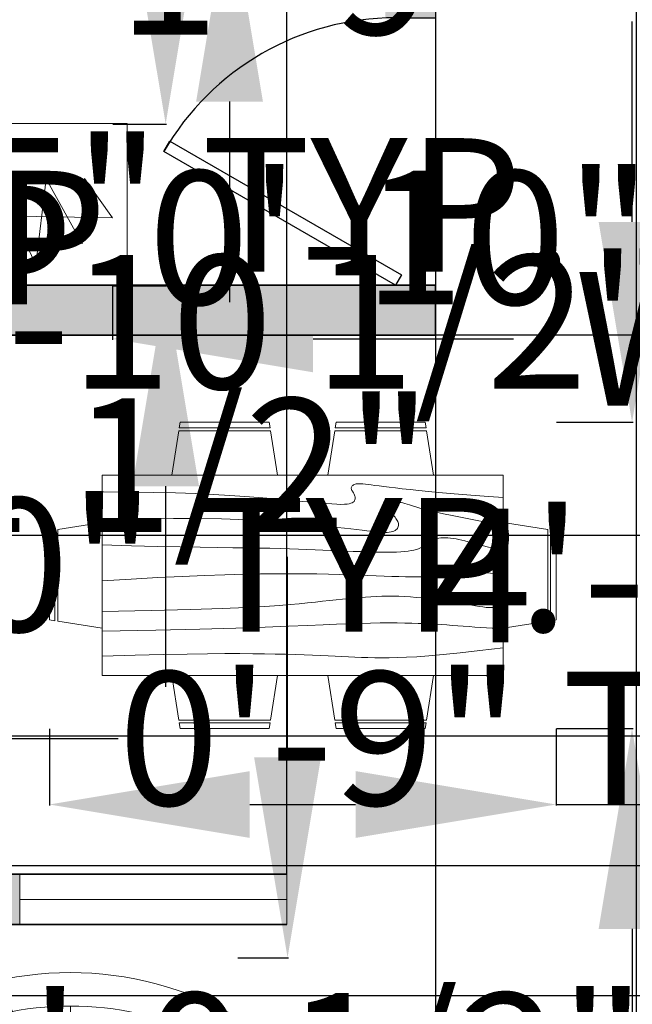
# Model space of a CAD drawing. Units: inches. Extents: x 2838 to 4029, y 1041 to 1915.
# Tile 6 of 16: x 3331 to 3441, y 1377 to 1554. Entities that reach past the tile are written whole.
import ezdxf

# ---------------------------------------------------------------- set-up
doc = ezdxf.new("R2010")
doc.units = ezdxf.units.IN
doc.header["$MEASUREMENT"] = 0
for name, color, linetype, lineweight in [('A-ANNO-DIMS', 2, 'Continuous', 18), ('A-DOOR', 3, 'Continuous', 25), ('A-FLOR-CASE', 8, 'Continuous', 18), ('A-FURN', 8, 'Continuous', 18), ('A-GLAZ', 4, 'Continuous', 18), ('A-WALL', 7, 'Continuous', 35), ('A-WALL-PATT', 252, 'Continuous', 13)]:
    doc.layers.add(name, color=color, linetype=linetype, lineweight=lineweight)
doc.styles.get("Standard").update_dxf_attribs({"font": 'arial.ttf'})
doc.dimstyles.get("Standard").update_dxf_attribs({"dimtxt": 24, "dimasz": 36, "dimexe": 0.18, "dimexo": 0.0625, "dimgap": 0.09, "dimtad": 0, "dimtih": 1, "dimtoh": 1, "dimdec": 0, "dimzin": 0, "dimdsep": 46, "dimlunit": 3, "dimtxsty": 'Standard', "dimcen": 0.09, "dimadec": 0, "dimazin": 0, "dimtfac": 1, "dimtdec": 0, "dimtofl": 0, "dimtmove": 0, "dimatfit": 3, "dimfxl": 1, "dimtolj": 1, "dimtzin": 0, "dimarcsym": 0})

# ---------------------------------------------------------------- blocks, each defined once
blk = doc.blocks.new('*U3')
for p, q in [((-40, 0), (-40, 6)), ((0, 0), (0, 6))]:
    blk.add_line(p, q)
blk.add_lwpolyline([(0, 0), (-20, -34.64), (-21.52, -33.77), (-1.52, 0.88)], close=True)
blk.add_arc((0, 0), 40, 180, 240)
blk = doc.blocks.new('Sofa - Roundback Loveseat 5 ft.')
for p, q in [((0, -32.44198), (0, -5.99998)), ((-24, -33.99998), (-24, -11.46958)), ((24.00004, -33.99998), (24.00004, -11.46958)), ((-23.9998, -13.38178), (23.99986, -13.38178)), ((-24, -32.44198), (24.00004, -32.44198))]:
    blk.add_line(p, q)
for points in [[(-24, -33.99998), (-30, -33.99998), (-30, -7.99998)], [(30.00004, -7.99998), (30.00004, -33.99998), (24.00004, -33.99998)]]:
    blk.add_lwpolyline(points)
for centre, radius, start, end in [((0, -60.24998), 60.24998, 60.13715, 119.8628), ((0, -61.38438), 55.38444, 64.32083, 115.6792)]:
    blk.add_arc(centre, radius, start, end)
blk = doc.blocks.new('Dining Set - 36 x 72 in.')
for p, q in [((-22, 27.5), (-22.1562, 26.50042)), ((-22, 27.5), (-6, 27.5)), ((-5.8437, 26.49966), (-6, 27.5)), ((6, 27.5), (5.8438, 26.50042)), ((6, 27.5), (22, 27.5)), ((22.1563, 26.49966), (22, 27.5)), ((-22.2343, 26.00059), (-23.4847, 17.99762)), ((-22.2304, 26), (-5.7608, 26)), ((-5.8416, 26.5), (-22.1534, 26.5)), ((-4.5152, 17.99762), (-5.7655, 25.99926)), ((5.7657, 26.00059), (4.5153, 17.99762)), ((5.7696, 26), (22.2392, 26)), ((22.1584, 26.5), (5.8466, 26.5)), ((23.4848, 17.99762), (22.2345, 25.99926)), ((36, 18), (-36, 18)), ((-36, 18), (-36, -18)), ((36, -18), (36, 18)), ((-44.0006, 8.23428), (-35.9976, 9.48474)), ((44.0006, 8.23428), (35.9976, 9.48474)), ((-45.5, 8), (-44.5004, 8.15617)), ((-45.5, 8), (-45.5, -8)), ((-44.5, -8.15843), (-44.5, 8.15338)), ((-44, 8.23041), (-44, -8.23915)), ((44, 8.23041), (44, -8.23915)), ((44.5, -8.15843), (44.5, 8.15338)), ((45.5, 8), (44.5005, 8.15617)), ((45.5, 8), (45.5, -8)), ((-44.4997, -8.15631), (-45.5, -8)), ((-35.9976, -9.48476), (-43.9993, -8.2345)), ((35.9976, -9.48476), (43.9993, -8.2345)), ((44.4997, -8.15631), (45.5, -8)), ((-36, -18), (36, -18)), ((-22.2343, -26.0006), (-23.4847, -17.99762)), ((-4.5152, -17.99762), (-5.7655, -25.99928)), ((5.7657, -26.0006), (4.5153, -17.99762)), ((23.4848, -17.99762), (22.2345, -25.99928)), ((-22.2304, -26), (-5.7608, -26)), ((-22, -27.5), (-22.1562, -26.50044)), ((-5.8416, -26.5), (-22.1534, -26.5)), ((-5.8437, -26.49967), (-6, -27.5)), ((5.7696, -26), (22.2392, -26)), ((6, -27.5), (5.8438, -26.50044)), ((22.1584, -26.5), (5.8466, -26.5)), ((22.1563, -26.49967), (22, -27.5)), ((-22, -27.5), (-6, -27.5)), ((6, -27.5), (22, -27.5))]:
    blk.add_line(p, q)
for points in [[(-36, 15), (-31.1772, 14.97754), (-26.8079, 14.91406), (-22.8538, 14.81543), (-19.276, 14.6875), (-16.0362, 14.53613), (-13.0957, 14.36718), (-10.4159, 14.18652), (-7.9583, 14), (-5.6904, 13.81315), (-3.6035, 13.63021), (-1.6954, 13.45508), (0.0365, 13.29166), (1.5945, 13.14388), (2.9811, 13.01562), (4.1988, 12.9108), (5.25, 12.83333), (6.1393, 12.78613), (6.8802, 12.76823), (7.4883, 12.77767), (7.9792, 12.8125), (8.3685, 12.87077), (8.6719, 12.95052), (8.9049, 13.0498), (9.0833, 13.16666), (9.2205, 13.29899), (9.3216, 13.44401), (9.3895, 13.59879), (9.4271, 13.76041), (9.4373, 13.92594), (9.4232, 14.09245), (9.3875, 14.257), (9.3333, 14.41666), (9.2638, 14.56917), (9.1836, 14.71484), (9.0975, 14.85465), (9.0104, 14.98958), (8.9272, 15.1206), (8.8529, 15.2487), (8.7922, 15.37483), (8.75, 15.5), (8.7305, 15.62467), (8.7344, 15.74739), (8.7617, 15.86621), (8.8125, 15.97916), (8.8867, 16.08431), (8.9844, 16.17968), (9.1055, 16.26334), (9.25, 16.33333), (9.4189, 16.38802), (9.6172, 16.42708), (9.8506, 16.45052), (10.125, 16.45833), (10.4463, 16.45052), (10.8203, 16.42708), (11.2529, 16.38802), (11.75, 16.33333), (12.3184, 16.26318), (12.9694, 16.17838), (13.7151, 16.07991), (14.5677, 15.96875), (15.5395, 15.84586), (16.6426, 15.71224), (17.8893, 15.56884), (19.2917, 15.41666), (20.859, 15.25667), (22.5879, 15.08984), (24.4721, 14.91715), (26.5052, 14.73958), (28.6809, 14.5581), (30.9929, 14.3737), (33.4347, 14.18733), (36, 14)], [(-36, 10), (-28.9766, 10.14274), (-23.1725, 10.20442), (-18.4241, 10.19775), (-14.5677, 10.13541), (-11.4399, 10.03011), (-8.877, 9.89453), (-6.7154, 9.74137), (-4.7917, 9.58333), (-2.9698, 9.43082), (-1.2246, 9.28515), (0.4415, 9.14534), (2.026, 9.01041), (3.5266, 8.87939), (4.9408, 8.7513), (6.266, 8.62516), (7.5, 8.5), (8.6411, 8.37549), (9.6914, 8.2539), (10.6538, 8.13818), (11.5312, 8.03125), (12.3267, 7.93603), (13.043, 7.85547), (13.6831, 7.79248), (14.25, 7.75), (14.7471, 7.7303), (15.1797, 7.73307), (15.5537, 7.75732), (15.875, 7.80208), (16.1494, 7.86637), (16.3828, 7.94922), (16.5811, 8.04964), (16.75, 8.16666), (16.8944, 8.29915), (17.0143, 8.44531), (17.1089, 8.60319), (17.1771, 8.77083), (17.218, 8.94629), (17.2305, 9.1276), (17.2137, 9.31282), (17.1667, 9.5), (17.0895, 9.6875), (16.987, 9.875), (16.8649, 10.0625), (16.7292, 10.25), (16.5856, 10.4375), (16.4401, 10.625), (16.2985, 10.8125), (16.1667, 11), (16.05, 11.18733), (15.9518, 11.3737), (15.8752, 11.5581), (15.8229, 11.73958), (15.798, 11.91715), (15.8034, 12.08984), (15.842, 12.25667), (15.9167, 12.41666), (16.0295, 12.56836), (16.1784, 12.70833), (16.3605, 12.83268), (16.5729, 12.9375), (16.8127, 13.01888), (17.0768, 13.07291), (17.3625, 13.0957), (17.6667, 13.08333), (17.9894, 13.03312), (18.3418, 12.94726), (18.7382, 12.82918), (19.1927, 12.68229), (19.7195, 12.51001), (20.3327, 12.31575), (21.0465, 12.10294), (21.875, 11.875), (22.8357, 11.63354), (23.959, 11.37304), (25.2786, 11.08618), (26.8282, 10.76562), (28.6414, 10.40405), (30.752, 9.99414), (33.1936, 9.52856), (36, 9)], [(-36, 5.5), (-30.7157, 5.3348), (-26.069, 5.20963), (-21.9946, 5.11767), (-18.4271, 5.05208), (-15.3009, 5.00602), (-12.5508, 4.97265), (-10.1112, 4.94515), (-7.9167, 4.91666), (-5.909, 4.88167), (-4.0586, 4.83984), (-2.3429, 4.79215), (-0.7396, 4.73958), (0.7739, 4.6831), (2.22, 4.6237), (3.6213, 4.56233), (5, 4.5), (6.373, 4.43782), (7.7344, 4.3776), (9.0723, 4.32129), (10.375, 4.27083), (11.6309, 4.22819), (12.8281, 4.19531), (13.9551, 4.17415), (15, 4.16666), (15.954, 4.17448), (16.819, 4.19791), (17.6001, 4.23698), (18.3021, 4.29166), (18.9299, 4.36198), (19.4883, 4.44791), (19.9823, 4.54948), (20.4167, 4.66666), (20.7969, 4.79899), (21.1302, 4.94401), (21.4245, 5.09879), (21.6875, 5.26041), (21.9271, 5.42594), (22.1511, 5.59245), (22.3672, 5.757), (22.5834, 5.91666), (22.8065, 6.06868), (23.0404, 6.21093), (23.2879, 6.34147), (23.5521, 6.45833), (23.8358, 6.55957), (24.142, 6.64323), (24.4735, 6.70735), (24.8334, 6.75), (25.2235, 6.76969), (25.642, 6.76692), (26.0858, 6.74267), (26.5521, 6.69791), (27.0379, 6.63362), (27.5404, 6.55078), (28.0565, 6.45036), (28.5834, 6.33333), (29.1242, 6.19987), (29.7071, 6.04687), (30.3661, 5.87044), (31.1354, 5.66666), (32.0493, 5.43164), (33.142, 5.16146), (34.4475, 4.85221), (36, 4.5)], [(-36, -1), (-30.7915, -0.6591), (-26.0195, -0.38216), (-21.6519, -0.16284), (-17.6563, 0.00521), (-14.0005, 0.12833), (-10.6523, 0.21289), (-7.5796, 0.26522), (-4.75, 0.29166), (-2.134, 0.29793), (0.2878, 0.28711), (2.5317, 0.26163), (4.6146, 0.22396), (6.5529, 0.17651), (8.3633, 0.12174), (10.0623, 0.06209), (11.6667, 0), (13.1899, -0.06201), (14.6341, -0.1211), (15.9982, -0.17432), (17.2813, -0.21875), (18.4823, -0.25147), (19.6003, -0.26953), (20.6343, -0.27002), (21.5834, -0.25), (22.4481, -0.20768), (23.2357, -0.14584), (23.9549, -0.06836), (24.6146, 0.02083), (25.2235, 0.11784), (25.7904, 0.21875), (26.3241, 0.31966), (26.8334, 0.41666), (27.3265, 0.50618), (27.8099, 0.58593), (28.2894, 0.65397), (28.7709, 0.70833), (29.2601, 0.74707), (29.763, 0.76823), (30.2855, 0.76985), (30.8334, 0.75), (31.4088, 0.70784), (31.9994, 0.64713), (32.589, 0.57275), (33.1615, 0.48958), (33.7008, 0.4025), (34.1908, 0.3164), (34.6153, 0.23616), (34.9584, 0.16666), (35.2099, 0.11165), (35.3848, 0.07031), (35.504, 0.04069), (35.5886, 0.02083), (35.6594, 0.00879), (35.7377, 0.0026), (35.8442, 0.00032), (36, 0)], [(-36, -6.5), (-27.1843, -6.31267), (-20.084, -6.1263), (-14.469, -5.9419), (-10.1094, -5.76042), (-6.7752, -5.58285), (-4.2363, -5.41016), (-2.2629, -5.24333), (-0.625, -5.08334), (0.8708, -4.93099), (2.2715, -4.78646), (3.5872, -4.64974), (4.8281, -4.52084), (6.0046, -4.39974), (7.127, -4.28646), (8.2053, -4.18099), (9.25, -4.08334), (10.2705, -3.99382), (11.2734, -3.91407), (12.2647, -3.84603), (13.25, -3.79167), (14.2354, -3.75293), (15.2266, -3.73177), (16.2295, -3.73015), (17.25, -3.75), (18.2912, -3.79248), (19.3451, -3.85547), (20.4009, -3.93604), (21.4479, -4.03125), (22.4754, -4.13819), (23.4727, -4.25391), (24.4289, -4.37549), (25.3334, -4.5), (26.1785, -4.62492), (26.9694, -4.74935), (27.7145, -4.87281), (28.4219, -4.99479), (29.1, -5.11483), (29.7572, -5.23242), (30.4016, -5.34709), (31.0417, -5.45834), (31.6837, -5.56437), (32.3262, -5.65821), (32.9658, -5.73153), (33.599, -5.77604), (34.2224, -5.78345), (34.8327, -5.74545), (35.4264, -5.65373), (36, -5.5)], [(-36, -10), (-26.4022, -9.81299), (-18.4675, -9.62891), (-11.9839, -9.45069), (-6.7396, -9.28125), (-2.5226, -9.12354), (0.8789, -8.98047), (3.6769, -8.85498), (6.0833, -8.75), (8.2767, -8.66765), (10.3021, -8.60677), (12.1712, -8.56543), (13.8958, -8.54167), (15.4876, -8.53353), (16.9583, -8.53907), (18.3197, -8.55632), (19.5834, -8.58334), (20.7616, -8.61841), (21.8685, -8.66081), (22.9188, -8.71004), (23.9271, -8.76563), (24.9081, -8.82707), (25.8763, -8.89388), (26.8465, -8.96558), (27.8334, -9.04167), (28.8474, -9.12118), (29.8828, -9.20117), (30.93, -9.27824), (31.9792, -9.34896), (33.0205, -9.40991), (34.0443, -9.45768), (35.0407, -9.48885), (36, -9.5)], [(-36, -14.5), (-30.0881, -14.33513), (-25.0332, -14.21224), (-20.7312, -14.12647), (-17.0781, -14.07292), (-13.97, -14.04671), (-11.3027, -14.04297), (-8.9724, -14.05681), (-6.875, -14.08334), (-4.9224, -14.11833), (-3.0905, -14.16016), (-1.3709, -14.20785), (0.2448, -14.26042), (1.7647, -14.3169), (3.1973, -14.3763), (4.5507, -14.43767), (5.8333, -14.5), (7.0554, -14.5621), (8.235, -14.62175), (9.3922, -14.67652), (10.5469, -14.72396), (11.7192, -14.76164), (12.929, -14.78711), (14.1965, -14.79794), (15.5417, -14.79167), (16.9933, -14.76424), (18.6152, -14.70508), (20.4804, -14.60197), (22.6615, -14.44271), (25.2312, -14.21509), (28.2624, -13.9069), (31.8277, -13.50594), (36, -13)]]:
    blk.add_lwpolyline(points)
blk = doc.blocks.new('WIN-48')
blk.add_line((4.5, 48), (4.5, 0))
blk.add_lwpolyline([(0, 48), (9, 48), (9, 0), (0, 0)], close=True)
blk = doc.blocks.new('WARDROBE-RAIL')
for p, q in [((1.86, 0), (12.76, 29.05)), ((12.76, 29.05), (12.76, 0)), ((12.76, 0), (20.9, 24.31)), ((20.9, 24.31), (26.94, 1.83)), ((26.94, 1.83), (31.9, 21.29)), ((31.9, 21.29), (40.3, 2.75)), ((40.3, 2.75), (41.22, 21.97)), ((41.22, 21.97), (49.7, 3.76)), ((1.8, 18), (1.86, 0)), ((49.7, 3.76), (51.56, 19.2)), ((51.56, 19.2), (58.03, 7.54)), ((58.03, 7.54), (58.45, 19.29)), ((58.45, 19.29), (63.49, 12.24)), ((63.49, 12.24), (0, 13.24)), ((0, 13.24), (63.49, 12.24))]:
    blk.add_line(p, q)
blk = doc.blocks.new('*D25')
at = {"layer": 'A-ANNO-DIMS', "color": 0, "lineweight": -2, "transparency": 16777216}
for p, q in [((3283.93, 1516.17), (3283.93, 1552.17)), ((3276.79, 1480.17), (3284.11, 1480.17)), ((3276.79, 1432.17), (3284.11, 1432.17)), ((3283.93, 1396.17), (3283.93, 1360.17))]:
    blk.add_line(p, q, dxfattribs=at)
at = {"layer": 'A-ANNO-DIMS', "color": 0, "transparency": 16777216}
for points in [[(3277.93, 1516.17), (3289.93, 1516.17), (3283.93, 1480.17)], [(3277.93, 1396.17), (3289.93, 1396.17), (3283.93, 1432.17)]]:
    blk.add_solid(points, dxfattribs=at)
at = {"layer": 'Defpoints', "color": 0, "transparency": 16777216}
for p in [(3276.73, 1480.17), (3283.93, 1480.17), (3276.73, 1432.17)]:
    blk.add_point(p, dxfattribs=at)
at = {"layer": 'A-ANNO-DIMS', "color": 0, "transparency": 16777216, "insert": (3283.93, 1456.17), "char_height": 24, "attachment_point": 5}
blk.add_mtext('\\A1;WINDOW 4\'-0" TYP.', dxfattribs=at)
blk = doc.blocks.new('*D26')
at = {"layer": 'A-ANNO-DIMS', "color": 0, "lineweight": -2, "transparency": 16777216}
for p, q in [((3267.73, 1432.1), (3267.73, 1424.79)), ((3276.73, 1432.1), (3276.73, 1424.79)), ((3231.73, 1424.97), (3195.73, 1424.97)), ((3312.73, 1424.97), (3348.73, 1424.97))]:
    blk.add_line(p, q, dxfattribs=at)
at = {"layer": 'A-ANNO-DIMS', "color": 0, "transparency": 16777216}
for points in [[(3231.73, 1430.97), (3231.73, 1418.97), (3267.73, 1424.97)], [(3312.73, 1430.97), (3312.73, 1418.97), (3276.73, 1424.97)]]:
    blk.add_solid(points, dxfattribs=at)
at = {"layer": 'Defpoints', "color": 0, "transparency": 16777216}
for p in [(3267.73, 1432.17), (3276.73, 1432.17), (3276.73, 1424.97)]:
    blk.add_point(p, dxfattribs=at)
at = {"layer": 'A-ANNO-DIMS', "color": 0, "transparency": 16777216, "insert": (3421.97, 1424.97), "char_height": 24, "attachment_point": 5}
blk.add_mtext('\\A1;0\'-9" TYP.', dxfattribs=at)
blk = doc.blocks.new('*D30')
at = {"layer": 'A-ANNO-DIMS', "color": 0, "lineweight": -2, "transparency": 16777216}
for p, q in [((3379.15, 1421.58), (3379.15, 1457.58)), ((3370.21, 1385.58), (3379.33, 1385.58)), ((3370.21, 1348.91), (3379.33, 1348.91)), ((3379.15, 1312.91), (3379.15, 1276.91))]:
    blk.add_line(p, q, dxfattribs=at)
at = {"layer": 'A-ANNO-DIMS', "color": 0, "transparency": 16777216}
for points in [[(3373.15, 1421.58), (3385.15, 1421.58), (3379.15, 1385.58)], [(3373.15, 1312.91), (3385.15, 1312.91), (3379.15, 1348.91)]]:
    blk.add_solid(points, dxfattribs=at)
at = {"layer": 'Defpoints', "color": 0, "transparency": 16777216}
for p in [(3370.15, 1385.58), (3379.15, 1385.58), (3370.15, 1348.91)]:
    blk.add_point(p, dxfattribs=at)
at = {"layer": 'A-ANNO-DIMS', "color": 0, "transparency": 16777216, "insert": (3379.15, 1367.25), "char_height": 24, "attachment_point": 5}
blk.add_mtext('\\A1;3\'-0 1/2"', dxfattribs=at)
blk = doc.blocks.new('*D33')
at = {"layer": 'A-ANNO-DIMS', "color": 0, "lineweight": -2, "transparency": 16777216}
for p, q in [((3601.73, 1469.45), (3601.73, 1505.45)), ((3603.48, 1433.45), (3601.55, 1433.45)), ((3603.48, 1421.37), (3601.55, 1421.37)), ((3601.73, 1385.37), (3601.73, 1349.37)), ((3601.73, 1349.37), (3565.73, 1349.37))]:
    blk.add_line(p, q, dxfattribs=at)
at = {"layer": 'A-ANNO-DIMS', "color": 0, "transparency": 16777216}
for points in [[(3595.73, 1469.45), (3607.73, 1469.45), (3601.73, 1433.45)], [(3595.73, 1385.37), (3607.73, 1385.37), (3601.73, 1421.37)]]:
    blk.add_solid(points, dxfattribs=at)
at = {"layer": 'Defpoints', "color": 0, "transparency": 16777216}
for p in [(3603.54, 1433.45), (3601.73, 1421.37), (3603.54, 1421.37)]:
    blk.add_point(p, dxfattribs=at)
at = {"layer": 'A-ANNO-DIMS', "color": 0, "transparency": 16777216, "insert": (3496.18, 1349.37), "char_height": 24, "attachment_point": 5}
blk.add_mtext('\\A1;TAP 1\'-0"', dxfattribs=at)
blk = doc.blocks.new('*D35')
at = {"layer": 'A-ANNO-DIMS', "color": 0, "lineweight": -2, "transparency": 16777216}
for p, q in [((3480.45, 1632.93), (3480.45, 1668.93)), ((3481.89, 1596.93), (3480.27, 1596.93)), ((3481.89, 1586.93), (3480.27, 1586.93)), ((3480.45, 1550.93), (3480.45, 1514.93)), ((3480.45, 1514.93), (3444.45, 1514.93))]:
    blk.add_line(p, q, dxfattribs=at)
at = {"layer": 'A-ANNO-DIMS', "color": 0, "transparency": 16777216}
for points in [[(3474.45, 1632.93), (3486.45, 1632.93), (3480.45, 1596.93)], [(3474.45, 1550.93), (3486.45, 1550.93), (3480.45, 1586.93)]]:
    blk.add_solid(points, dxfattribs=at)
at = {"layer": 'Defpoints', "color": 0, "transparency": 16777216}
for p in [(3481.95, 1596.93), (3480.45, 1586.93), (3481.95, 1586.93)]:
    blk.add_point(p, dxfattribs=at)
at = {"layer": 'A-ANNO-DIMS', "color": 0, "transparency": 16777216, "insert": (3365.58, 1514.93), "char_height": 24, "attachment_point": 5}
blk.add_mtext('\\A1;TAP 0\'-10"', dxfattribs=at)
blk = doc.blocks.new('*D36')
at = {"layer": 'A-ANNO-DIMS', "color": 0, "lineweight": -2, "transparency": 16777216}
for p, q in [((3481.95, 1586.87), (3481.95, 1585.25)), ((3488.45, 1586.87), (3488.45, 1585.25)), ((3445.95, 1585.43), (3409.95, 1585.43)), ((3524.45, 1585.43), (3560.45, 1585.43))]:
    blk.add_line(p, q, dxfattribs=at)
at = {"layer": 'A-ANNO-DIMS', "color": 0, "transparency": 16777216}
for points in [[(3445.95, 1591.43), (3445.95, 1579.43), (3481.95, 1585.43)], [(3524.45, 1591.43), (3524.45, 1579.43), (3488.45, 1585.43)]]:
    blk.add_solid(points, dxfattribs=at)
at = {"layer": 'Defpoints', "color": 0, "transparency": 16777216}
for p in [(3481.95, 1586.93), (3488.45, 1586.93), (3488.45, 1585.43)]:
    blk.add_point(p, dxfattribs=at)
at = {"layer": 'A-ANNO-DIMS', "color": 0, "transparency": 16777216, "insert": (3620.4, 1585.43), "char_height": 24, "attachment_point": 5}
blk.add_mtext('\\A1;0\'-6 1/2"', dxfattribs=at)
blk = doc.blocks.new('*D38')
at = {"layer": 'A-ANNO-DIMS', "color": 0, "lineweight": -2, "transparency": 16777216}
for p, q in [((3368.73, 1671.36), (3368.73, 1707.36)), ((3356.79, 1635.36), (3368.91, 1635.36)), ((3356.79, 1575.36), (3368.91, 1575.36)), ((3368.73, 1539.36), (3368.73, 1503.36))]:
    blk.add_line(p, q, dxfattribs=at)
at = {"layer": 'A-ANNO-DIMS', "color": 0, "transparency": 16777216}
for points in [[(3362.73, 1671.36), (3374.73, 1671.36), (3368.73, 1635.36)], [(3362.73, 1539.36), (3374.73, 1539.36), (3368.73, 1575.36)]]:
    blk.add_solid(points, dxfattribs=at)
at = {"layer": 'Defpoints', "color": 0, "transparency": 16777216}
for p in [(3356.73, 1635.36), (3368.73, 1635.36), (3356.73, 1575.36)]:
    blk.add_point(p, dxfattribs=at)
at = {"layer": 'A-ANNO-DIMS', "color": 0, "transparency": 16777216, "insert": (3368.73, 1605.36), "char_height": 24, "attachment_point": 5}
blk.add_mtext('\\A1;5\'-0" TYP.', dxfattribs=at)
blk = doc.blocks.new('*D41')
at = {"layer": 'A-ANNO-DIMS', "color": 0, "lineweight": -2, "transparency": 16777216}
for p, q in [((3284.24, 1506.2), (3284.24, 1496.56)), ((3347.73, 1506.2), (3347.73, 1496.56)), ((3248.24, 1496.74), (3212.24, 1496.74)), ((3383.73, 1496.74), (3419.73, 1496.74))]:
    blk.add_line(p, q, dxfattribs=at)
at = {"layer": 'A-ANNO-DIMS', "color": 0, "transparency": 16777216}
for points in [[(3248.24, 1502.74), (3248.24, 1490.74), (3284.24, 1496.74)], [(3383.73, 1502.74), (3383.73, 1490.74), (3347.73, 1496.74)]]:
    blk.add_solid(points, dxfattribs=at)
at = {"layer": 'Defpoints', "color": 0, "transparency": 16777216}
for p in [(3284.24, 1506.26), (3347.73, 1506.26), (3347.73, 1496.74)]:
    blk.add_point(p, dxfattribs=at)
at = {"layer": 'A-ANNO-DIMS', "color": 0, "transparency": 16777216, "insert": (3624.81, 1496.74), "char_height": 24, "attachment_point": 5}
blk.add_mtext('\\A1;WARDROBE 5\'-3 1/2" TYP.', dxfattribs=at)
blk = doc.blocks.new('*D42')
at = {"layer": 'A-ANNO-DIMS', "color": 0, "lineweight": -2, "transparency": 16777216}
for p, q in [((3357.26, 1571.32), (3357.26, 1607.32)), ((3347.8, 1535.32), (3357.44, 1535.32)), ((3347.8, 1506.26), (3357.44, 1506.26)), ((3357.26, 1470.26), (3357.26, 1434.26))]:
    blk.add_line(p, q, dxfattribs=at)
at = {"layer": 'A-ANNO-DIMS', "color": 0, "transparency": 16777216}
for points in [[(3351.26, 1571.32), (3363.26, 1571.32), (3357.26, 1535.32)], [(3351.26, 1470.26), (3363.26, 1470.26), (3357.26, 1506.26)]]:
    blk.add_solid(points, dxfattribs=at)
at = {"layer": 'Defpoints', "color": 0, "transparency": 16777216}
for p in [(3347.73, 1535.32), (3357.26, 1535.32), (3347.73, 1506.26)]:
    blk.add_point(p, dxfattribs=at)
at = {"layer": 'A-ANNO-DIMS', "color": 0, "transparency": 16777216, "insert": (3357.26, 1520.79), "char_height": 24, "attachment_point": 5}
blk.add_mtext('\\A1;2\'-5" TYP.', dxfattribs=at)
blk = doc.blocks.new('*D46')
at = {"layer": 'A-ANNO-DIMS', "color": 0, "lineweight": -2, "transparency": 16777216}
for p, q in [((3451.73, 1692.41), (3451.73, 1728.41)), ((3456.62, 1656.41), (3451.55, 1656.41)), ((3456.62, 1635.41), (3451.55, 1635.41)), ((3451.73, 1599.41), (3451.73, 1563.41)), ((3451.73, 1563.41), (3415.73, 1563.41))]:
    blk.add_line(p, q, dxfattribs=at)
at = {"layer": 'A-ANNO-DIMS', "color": 0, "transparency": 16777216}
for points in [[(3445.73, 1692.41), (3457.73, 1692.41), (3451.73, 1656.41)], [(3445.73, 1599.41), (3457.73, 1599.41), (3451.73, 1635.41)]]:
    blk.add_solid(points, dxfattribs=at)
at = {"layer": 'Defpoints', "color": 0, "transparency": 16777216}
for p in [(3456.69, 1656.41), (3451.73, 1635.41), (3456.69, 1635.41)]:
    blk.add_point(p, dxfattribs=at)
at = {"layer": 'A-ANNO-DIMS', "color": 0, "transparency": 16777216, "insert": (3384.87, 1563.41), "char_height": 24, "attachment_point": 5}
blk.add_mtext('\\A1;1\'-9"', dxfattribs=at)
blk = doc.blocks.new('*D49')
at = {"layer": 'A-ANNO-DIMS', "color": 0, "lineweight": -2, "transparency": 16777216}
for p, q in [((3336.37, 1426.68), (3336.37, 1412.92)), ((3427.37, 1426.68), (3427.37, 1412.92)), ((3372.37, 1413.1), (3391.37, 1413.1)), ((3427.37, 1413.1), (3463.37, 1413.1))]:
    blk.add_line(p, q, dxfattribs=at)
at = {"layer": 'A-ANNO-DIMS', "color": 0, "transparency": 16777216}
for points in [[(3372.37, 1419.1), (3372.37, 1407.1), (3336.37, 1413.1)], [(3391.37, 1419.1), (3391.37, 1407.1), (3427.37, 1413.1)]]:
    blk.add_solid(points, dxfattribs=at)
at = {"layer": 'Defpoints', "color": 0, "transparency": 16777216}
for p in [(3336.37, 1426.75), (3427.37, 1426.75), (3427.37, 1413.1)]:
    blk.add_point(p, dxfattribs=at)
at = {"layer": 'A-ANNO-DIMS', "color": 0, "transparency": 16777216, "insert": (3595.36, 1413.1), "char_height": 24, "attachment_point": 5}
blk.add_mtext('\\A1;DINING SET 7\'-7"', dxfattribs=at)
blk = doc.blocks.new('*D50')
at = {"layer": 'A-ANNO-DIMS', "color": 0, "lineweight": -2, "transparency": 16777216}
for p, q in [((3441.02, 1517.75), (3441.02, 1553.75)), ((3427.44, 1481.75), (3441.2, 1481.75)), ((3427.44, 1426.75), (3441.2, 1426.75)), ((3441.02, 1390.75), (3441.02, 1354.75))]:
    blk.add_line(p, q, dxfattribs=at)
at = {"layer": 'A-ANNO-DIMS', "color": 0, "transparency": 16777216}
for points in [[(3435.02, 1517.75), (3447.02, 1517.75), (3441.02, 1481.75)], [(3435.02, 1390.75), (3447.02, 1390.75), (3441.02, 1426.75)]]:
    blk.add_solid(points, dxfattribs=at)
at = {"layer": 'Defpoints', "color": 0, "transparency": 16777216}
for p in [(3427.37, 1481.75), (3441.02, 1481.75), (3427.37, 1426.75)]:
    blk.add_point(p, dxfattribs=at)
at = {"layer": 'A-ANNO-DIMS', "color": 0, "transparency": 16777216, "insert": (3441.02, 1454.25), "char_height": 24, "attachment_point": 5}
blk.add_mtext('\\A1;4\'-7"', dxfattribs=at)
blk = doc.blocks.new('*D55')
at = {"layer": 'A-ANNO-DIMS', "color": 0, "lineweight": -2, "transparency": 16777216}
for p, q in [((3491.76, 1499.78), (3455.76, 1499.78)), ((3527.76, 1494.67), (3527.76, 1499.96)), ((3562.26, 1494.67), (3562.26, 1499.96)), ((3598.26, 1499.78), (3634.26, 1499.78))]:
    blk.add_line(p, q, dxfattribs=at)
at = {"layer": 'A-ANNO-DIMS', "color": 0, "transparency": 16777216}
for points in [[(3491.76, 1505.78), (3491.76, 1493.78), (3527.76, 1499.78)], [(3598.26, 1505.78), (3598.26, 1493.78), (3562.26, 1499.78)]]:
    blk.add_solid(points, dxfattribs=at)
at = {"layer": 'Defpoints', "color": 0, "transparency": 16777216}
for p in [(3527.76, 1499.78), (3527.76, 1494.6), (3562.26, 1494.6)]:
    blk.add_point(p, dxfattribs=at)
at = {"layer": 'A-ANNO-DIMS', "color": 0, "transparency": 16777216, "insert": (3260.33, 1499.78), "char_height": 24, "attachment_point": 5}
blk.add_mtext('\\A1;BASE CABINET 2\'-10 1/2"', dxfattribs=at)
blk = doc.blocks.new('*D73')
at = {"layer": 'A-ANNO-DIMS', "color": 0, "lineweight": -2, "transparency": 16777216}
for p, q in [((3425.038746, 1711.522346), (3389.038746, 1711.522346)), ((3461.038746, 1200.359846), (3461.038746, 1711.702346)), ((3618.731626, 1200.359846), (3618.731626, 1711.702346)), ((3654.731626, 1711.522346), (3690.731626, 1711.522346))]:
    blk.add_line(p, q, dxfattribs=at)
at = {"layer": 'A-ANNO-DIMS', "color": 0, "transparency": 16777216}
for points in [[(3425.038746, 1717.522346), (3425.038746, 1705.522346), (3461.038746, 1711.522346)], [(3654.731626, 1717.522346), (3654.731626, 1705.522346), (3618.731626, 1711.522346)]]:
    blk.add_solid(points, dxfattribs=at)
at = {"layer": 'Defpoints', "color": 0, "transparency": 16777216}
for p in [(3618.731626, 1711.522346), (3461.038746, 1200.297346), (3618.731626, 1200.297346)]:
    blk.add_point(p, dxfattribs=at)
at = {"layer": 'A-ANNO-DIMS', "color": 0, "transparency": 16777216, "insert": (3539.885186, 1711.522346), "char_height": 24, "attachment_point": 5}
blk.add_mtext('\\A1;13\'-1 1/2"', dxfattribs=at)
blk = doc.blocks.new('*D79')
at = {"layer": 'A-ANNO-DIMS', "color": 0, "lineweight": -2, "transparency": 16777216}
for p, q in [((3379.05, 1400.64), (3379.05, 1711.7)), ((3415.05, 1711.52), (3418.63, 1711.52)), ((3454.63, 1398.31), (3454.63, 1711.7)), ((3454.63, 1711.52), (3490.63, 1711.52))]:
    blk.add_line(p, q, dxfattribs=at)
at = {"layer": 'A-ANNO-DIMS', "color": 0, "transparency": 16777216}
for points in [[(3415.05, 1717.52), (3415.05, 1705.52), (3379.05, 1711.52)], [(3418.63, 1717.52), (3418.63, 1705.52), (3454.63, 1711.52)]]:
    blk.add_solid(points, dxfattribs=at)
at = {"layer": 'Defpoints', "color": 0, "transparency": 16777216}
for p in [(3454.63, 1711.52), (3379.05, 1400.57), (3454.63, 1398.25)]:
    blk.add_point(p, dxfattribs=at)
at = {"layer": 'A-ANNO-DIMS', "color": 0, "transparency": 16777216, "insert": (3550.65, 1711.52), "char_height": 24, "attachment_point": 5}
blk.add_mtext('\\A1;6\'-3 1/2"', dxfattribs=at)
blk = doc.blocks.new('*D82')
at = {"layer": 'A-ANNO-DIMS', "color": 0, "lineweight": -2, "transparency": 16777216}
for p, q in [((3405.73, 1573.06), (3405.73, 1081.89)), ((3441.73, 1569.23), (3441.73, 1081.89)), ((3369.73, 1082.07), (3333.73, 1082.07)), ((3477.73, 1082.07), (3513.73, 1082.07))]:
    blk.add_line(p, q, dxfattribs=at)
at = {"layer": 'A-ANNO-DIMS', "color": 0, "transparency": 16777216}
for points in [[(3369.73, 1088.07), (3369.73, 1076.07), (3405.73, 1082.07)], [(3477.73, 1088.07), (3477.73, 1076.07), (3441.73, 1082.07)]]:
    blk.add_solid(points, dxfattribs=at)
at = {"layer": 'Defpoints', "color": 0, "transparency": 16777216}
for p in [(3405.73, 1573.12), (3441.73, 1569.3), (3441.73, 1082.07)]:
    blk.add_point(p, dxfattribs=at)
at = {"layer": 'A-ANNO-DIMS', "color": 0, "transparency": 16777216, "insert": (3545.71, 1082.07), "char_height": 24, "attachment_point": 5}
blk.add_mtext('\\A1;3\'-0"', dxfattribs=at)
blk = doc.blocks.new('*D87')
at = {"layer": 'A-ANNO-DIMS', "color": 0, "lineweight": -2, "transparency": 16777216}
for p, q in [((3227.506626, 1497.394218), (3227.506626, 1533.394218)), ((3513.669126, 1461.394218), (3227.326626, 1461.394218)), ((3513.669126, 1425.394218), (3227.326626, 1425.394218)), ((3227.506626, 1389.394218), (3227.506626, 1353.394218))]:
    blk.add_line(p, q, dxfattribs=at)
at = {"layer": 'A-ANNO-DIMS', "color": 0, "transparency": 16777216}
for points in [[(3221.506626, 1497.394218), (3233.506626, 1497.394218), (3227.506626, 1461.394218)], [(3221.506626, 1389.394218), (3233.506626, 1389.394218), (3227.506626, 1425.394218)]]:
    blk.add_solid(points, dxfattribs=at)
at = {"layer": 'Defpoints', "color": 0, "transparency": 16777216}
for p in [(3227.506626, 1461.394218), (3513.731626, 1461.394218), (3513.731626, 1425.394218)]:
    blk.add_point(p, dxfattribs=at)
at = {"layer": 'A-ANNO-DIMS', "color": 0, "transparency": 16777216, "insert": (3227.506626, 1443.394218), "char_height": 24, "attachment_point": 5}
blk.add_mtext('\\A1;3\'-0"', dxfattribs=at)
blk = doc.blocks.new('*D91')
at = {"layer": 'A-ANNO-DIMS', "color": 0, "lineweight": -2, "transparency": 16777216}
for p, q in [((3227.506626, 1533.394218), (3227.506626, 1569.394218)), ((3522.669126, 1497.394218), (3227.326626, 1497.394218)), ((3522.669126, 1461.394218), (3227.326626, 1461.394218)), ((3227.506626, 1425.394218), (3227.506626, 1389.394218))]:
    blk.add_line(p, q, dxfattribs=at)
at = {"layer": 'A-ANNO-DIMS', "color": 0, "transparency": 16777216}
for points in [[(3221.506626, 1533.394218), (3233.506626, 1533.394218), (3227.506626, 1497.394218)], [(3221.506626, 1425.394218), (3233.506626, 1425.394218), (3227.506626, 1461.394218)]]:
    blk.add_solid(points, dxfattribs=at)
at = {"layer": 'Defpoints', "color": 0, "transparency": 16777216}
for p in [(3522.731626, 1497.394218), (3227.506626, 1461.394218), (3522.731626, 1461.394218)]:
    blk.add_point(p, dxfattribs=at)
at = {"layer": 'A-ANNO-DIMS', "color": 0, "transparency": 16777216, "insert": (3227.506626, 1479.394218), "char_height": 24, "attachment_point": 5}
blk.add_mtext('\\A1;3\'-0"', dxfattribs=at)
blk = doc.blocks.new('*D93')
at = {"layer": 'A-ANNO-DIMS', "color": 0, "lineweight": -2, "transparency": 16777216}
for p, q in [((3227.51, 1438.06), (3227.51, 1474.06)), ((3227.51, 1474.06), (3263.51, 1474.06)), ((3522.67, 1402.06), (3227.33, 1402.06)), ((3522.67, 1378.73), (3227.33, 1378.73)), ((3227.51, 1342.73), (3227.51, 1306.73))]:
    blk.add_line(p, q, dxfattribs=at)
at = {"layer": 'A-ANNO-DIMS', "color": 0, "transparency": 16777216}
for points in [[(3221.51, 1438.06), (3233.51, 1438.06), (3227.51, 1402.06)], [(3221.51, 1342.73), (3233.51, 1342.73), (3227.51, 1378.73)]]:
    blk.add_solid(points, dxfattribs=at)
at = {"layer": 'Defpoints', "color": 0, "transparency": 16777216}
for p in [(3227.51, 1402.06), (3522.73, 1402.06), (3522.73, 1378.73)]:
    blk.add_point(p, dxfattribs=at)
at = {"layer": 'A-ANNO-DIMS', "color": 0, "transparency": 16777216, "insert": (3331.65, 1474.06), "char_height": 24, "attachment_point": 5}
blk.add_mtext('\\A1;1\'-11 1/2"', dxfattribs=at)
blk = doc.blocks.new('*D101')
at = {"layer": 'A-ANNO-DIMS', "color": 0, "lineweight": -2, "transparency": 16777216}
for p, q in [((3425.04, 1711.52), (3389.04, 1711.52)), ((3461.04, 1200.36), (3461.04, 1711.7)), ((3486.18, 1200.36), (3486.18, 1711.7)), ((3522.18, 1711.52), (3558.18, 1711.52))]:
    blk.add_line(p, q, dxfattribs=at)
at = {"layer": 'A-ANNO-DIMS', "color": 0, "transparency": 16777216}
for points in [[(3425.04, 1717.52), (3425.04, 1705.52), (3461.04, 1711.52)], [(3522.18, 1717.52), (3522.18, 1705.52), (3486.18, 1711.52)]]:
    blk.add_solid(points, dxfattribs=at)
at = {"layer": 'Defpoints', "color": 0, "transparency": 16777216}
for p in [(3486.18, 1711.52), (3461.04, 1200.3), (3486.18, 1200.3)]:
    blk.add_point(p, dxfattribs=at)
at = {"layer": 'A-ANNO-DIMS', "color": 0, "transparency": 16777216, "insert": (3590.37, 1711.52), "char_height": 24, "attachment_point": 5}
blk.add_mtext('\\A1;2\'-1"', dxfattribs=at)
blk = doc.blocks.new('*D103')
at = {"layer": 'A-ANNO-DIMS', "color": 0, "lineweight": -2, "transparency": 16777216}
for p, q in [((3227.51, 1628.55), (3227.51, 1664.55)), ((3227.51, 1664.55), (3263.51, 1664.55)), ((3469.64, 1592.55), (3227.33, 1592.55)), ((3441.67, 1578.3), (3227.33, 1578.3)), ((3227.51, 1542.3), (3227.51, 1506.3))]:
    blk.add_line(p, q, dxfattribs=at)
at = {"layer": 'A-ANNO-DIMS', "color": 0, "transparency": 16777216}
for points in [[(3221.51, 1628.55), (3233.51, 1628.55), (3227.51, 1592.55)], [(3221.51, 1542.3), (3233.51, 1542.3), (3227.51, 1578.3)]]:
    blk.add_solid(points, dxfattribs=at)
at = {"layer": 'Defpoints', "color": 0, "transparency": 16777216}
for p in [(3227.51, 1592.55), (3469.7, 1592.55), (3441.73, 1578.3)]:
    blk.add_point(p, dxfattribs=at)
at = {"layer": 'A-ANNO-DIMS', "color": 0, "transparency": 16777216, "insert": (3322.33, 1664.55), "char_height": 24, "attachment_point": 5}
blk.add_mtext('\\A1;1\'-2 1/2"', dxfattribs=at)

msp = doc.modelspace()

# ---------------------------------------------------------------- hatches: boundary and pattern name
at = {"layer": 'A-WALL-PATT'}
h = msp.add_hatch(color=256, dxfattribs=at)
h.dxf.hatch_style = 1
h.paths.add_polyline_path([(3405.73, 1506.39), (3297.05, 1506.39), (3297.01, 1506.26), (3297.01, 1506.39), (3286.16, 1506.39), (3286.11, 1506.26), (3286.11, 1506.39), (3276.73, 1506.39), (3276.73, 1535.45), (3276.73, 1662.3), (3312.91, 1662.3), (3312.91, 1671.3), (3267.73, 1671.3), (3267.73, 1480.17), (3276.73, 1480.17), (3276.73, 1497.39), (3405.73, 1497.39)])
h = msp.add_hatch(color=256, dxfattribs=at)
h.dxf.hatch_style = 1
h.paths.add_polyline_path([(3427.52, 1671.3), (3360.91, 1671.3), (3360.91, 1662.3), (3396.73, 1662.3), (3396.73, 1554.39), (3397.12, 1554.39, -0.007312), (3398.53, 1554.41), (3405.73, 1554.41), (3405.73, 1662.3), (3427.52, 1662.3)])
h.paths.add_polyline_path([(3546.42, 1671.3), (3451.52, 1671.3), (3451.52, 1662.3), (3489.73, 1662.3), (3489.73, 1592.86, -0.016107), (3489.73, 1591.9), (3489.73, 1578.3), (3441.73, 1578.3), (3441.73, 1569.3), (3489.73, 1569.3), (3489.73, 1554.41), (3498.73, 1554.41), (3498.73, 1662.3), (3546.42, 1662.3)])
h.paths.add_polyline_path([(3627.73, 1671.3), (3594.42, 1671.3), (3594.42, 1662.3), (3618.73, 1662.3), (3618.73, 1634.03), (3627.73, 1634.03)])
h.paths.add_polyline_path([(3627.73, 1586.03), (3618.73, 1586.03), (3618.73, 1506.39), (3545.12, 1506.39), (3489.73, 1506.39), (3489.73, 1497.39), (3513.73, 1497.39), (3618.73, 1497.39), (3618.73, 1469.85), (3627.73, 1469.85)])
h.paths.add_polyline_path([(3627.73, 1421.85), (3618.73, 1421.85), (3618.73, 1378.73), (3522.73, 1378.73), (3513.73, 1378.73), (3461.04, 1378.73), (3461.04, 1369.73), (3513.73, 1369.73), (3618.73, 1369.73), (3618.73, 1320.94), (3627.73, 1320.94)])
h.paths.add_polyline_path([(3627.73, 1272.94), (3618.73, 1272.94), (3618.73, 1200.3), (3599.07, 1200.3), (3599.07, 1191.3), (3627.73, 1191.3)])
h.paths.add_polyline_path([(3551.07, 1200.3), (3510.18, 1200.3), (3510.18, 1191.3), (3551.07, 1191.3)])
h.paths.add_polyline_path([(3486.18, 1200.3), (3461.04, 1200.3), (3461.04, 1398.25), (3454.63, 1398.25), (3454.63, 1200.3), (3432.45, 1200.3), (3432.45, 1191.3), (3486.18, 1191.3)])
h.paths.add_polyline_path([(3300.73, 1200.3), (3276.73, 1200.3), (3276.73, 1391.57), (3331.05, 1391.57), (3331.05, 1400.57), (3276.73, 1400.57), (3276.73, 1432.17), (3267.73, 1432.17), (3267.73, 1191.3), (3300.73, 1191.3)])

# ---------------------------------------------------------------- linework, layer by layer
at = {"layer": 'A-FLOR-CASE'}
msp.add_lwpolyline([(3276.73, 1535.45), (3350.34, 1535.45), (3350.34, 1506.39), (3276.73, 1506.39)], close=True, dxfattribs=at)
at = {"layer": 'A-WALL'}
for p, q in [((3405.73, 1506.39), (3276.73, 1506.39)), ((3405.73, 1506.39), (3276.73, 1506.39)), ((3405.73, 1506.39), (3405.73, 1497.39)), ((3405.73, 1497.39), (3405.73, 1506.39)), ((3405.73, 1497.39), (3276.73, 1497.39)), ((3276.73, 1497.39), (3405.73, 1497.39)), ((3379.05, 1400.57), (3276.73, 1400.57)), ((3379.05, 1400.57), (3276.73, 1400.57)), ((3379.05, 1391.57), (3276.73, 1391.57)), ((3379.05, 1391.57), (3276.73, 1391.57))]:
    msp.add_line(p, q, dxfattribs=at)

# ---------------------------------------------------------------- block references
at = {"layer": 'A-DOOR', "xscale": 1.200513446172712, "yscale": 1.200513446172712, "zscale": 1.200513446172712, "rotation": 270}
msp.add_blockref('*U3', (3398.53, 1506.39), dxfattribs=at)
at = {"layer": 'A-FLOR-CASE'}
msp.add_blockref('WARDROBE-RAIL', (3284.24, 1506.26), dxfattribs=at)
at = {"layer": 'A-FURN'}
for name, p in [('Dining Set - 36 x 72 in.', (3381.87, 1454.25)), ('Sofa - Roundback Loveseat 5 ft.', (3340.15, 1382.91))]:
    msp.add_blockref(name, p, dxfattribs=at)
at = {"layer": 'A-GLAZ', "rotation": 269.9999999999966}
msp.add_blockref('WIN-48', (3331.05, 1400.57), dxfattribs=at)

# ---------------------------------------------------------------- dimensions: what is measured, and where the dimension line sits
at = {"layer": 'A-ANNO-DIMS'}
for base, p1, p2, picture, middle in [((3454.63, 1711.52), (3379.05, 1400.57), (3454.63, 1398.25), '*D79', (3550.65, 1711.52)), ((3618.73, 1711.52), (3461.04, 1200.3), (3618.73, 1200.3), '*D73', (3539.89, 1711.52)), ((3486.18, 1711.52), (3461.04, 1200.3), (3486.18, 1200.3), '*D101', (3590.37, 1711.52)), ((3488.45, 1585.43), (3481.95, 1586.93), (3488.45, 1586.93), '*D36', (3620.4, 1585.43)), ((3441.73, 1082.07), (3405.73, 1573.12), (3441.73, 1569.3), '*D82', (3545.71, 1082.07))]:
    dim = msp.add_linear_dim(base=base, p1=p1, p2=p2, dimstyle='Standard', override={"dimdec": 1, "dimlfac": 1, "dimrnd": 0, "dimzin": 1, "dimdsep": 46, "dimlunit": 4, "dimfrac": 2}, dxfattribs=at)
    dim.commit()
    dim.dimension.update_dxf_attribs({"geometry": picture, "text_midpoint": middle})
for base, p1, p2, angle, picture, middle in [((3451.73, 1635.41), (3456.69, 1656.41), (3456.69, 1635.41), 270, '*D46', (3384.87, 1563.41)), ((3227.5066, 1592.5486), (3441.7316, 1578.2973), (3469.6999, 1592.5486), 90, '*D103', (3322.3279, 1664.5486)), ((3227.51, 1461.39), (3522.73, 1497.39), (3522.73, 1461.39), 90, '*D91', (3227.51, 1479.39)), ((3441.02, 1481.75), (3427.37, 1426.75), (3427.37, 1481.75), 90, '*D50', (3441.02, 1454.25)), ((3227.51, 1461.39), (3513.73, 1425.39), (3513.73, 1461.39), 90, '*D87', (3227.51, 1443.39)), ((3227.51, 1402.06), (3522.73, 1378.73), (3522.73, 1402.06), 90, '*D93', (3331.65, 1474.06)), ((3379.15, 1385.58), (3370.15, 1348.91), (3370.15, 1385.58), 90, '*D30', (3379.15, 1367.25))]:
    dim = msp.add_linear_dim(base=base, p1=p1, p2=p2, angle=angle, dimstyle='Standard', override={"dimdec": 1, "dimlfac": 1, "dimrnd": 0, "dimzin": 1, "dimdsep": 46, "dimlunit": 4, "dimfrac": 2}, dxfattribs=at)
    dim.commit()
    dim.dimension.update_dxf_attribs({"geometry": picture, "text_midpoint": middle})
for base, p1, p2, angle, text, picture, middle in [((3368.73, 1635.36), (3356.73, 1575.36), (3356.73, 1635.36), 90, '<> TYP.', '*D38', (3368.73, 1605.36)), ((3480.45, 1586.93), (3481.95, 1596.93), (3481.95, 1586.93), 270, 'TAP <>', '*D35', (3365.58, 1514.93)), ((3357.26, 1535.32), (3347.73, 1506.26), (3347.73, 1535.32), 90, '<> TYP.', '*D42', (3357.26, 1520.79)), ((3527.76, 1499.78), (3562.26, 1494.6), (3527.76, 1494.6), 180, 'BASE CABINET <>', '*D55', (3260.33, 1499.78)), ((3283.93, 1480.17), (3276.73, 1432.17), (3276.73, 1480.17), 90, 'WINDOW <> TYP.', '*D25', (3283.93, 1456.17)), ((3601.73, 1421.37), (3603.54, 1433.45), (3603.54, 1421.37), 270, 'TAP <>', '*D33', (3496.18, 1349.37))]:
    dim = msp.add_linear_dim(base=base, p1=p1, p2=p2, angle=angle, text=text, dimstyle='Standard', override={"dimdec": 1, "dimlfac": 1, "dimrnd": 0, "dimzin": 1, "dimdsep": 46, "dimlunit": 4, "dimfrac": 2}, dxfattribs=at)
    dim.commit()
    dim.dimension.update_dxf_attribs({"geometry": picture, "text_midpoint": middle})
for base, p1, p2, text, picture, middle in [((3347.73, 1496.74), (3284.24, 1506.26), (3347.73, 1506.26), 'WARDROBE <> TYP.', '*D41', (3624.81, 1496.74)), ((3427.37, 1413.1), (3336.37, 1426.75), (3427.37, 1426.75), 'DINING SET <>', '*D49', (3595.36, 1413.1)), ((3276.73, 1424.97), (3267.73, 1432.17), (3276.73, 1432.17), '<> TYP.', '*D26', (3421.97, 1424.97))]:
    dim = msp.add_linear_dim(base=base, p1=p1, p2=p2, text=text, dimstyle='Standard', override={"dimdec": 1, "dimlfac": 1, "dimrnd": 0, "dimzin": 1, "dimdsep": 46, "dimlunit": 4, "dimfrac": 2}, dxfattribs=at)
    dim.commit()
    dim.dimension.update_dxf_attribs({"geometry": picture, "text_midpoint": middle})

doc.saveas('drawing.dxf')
